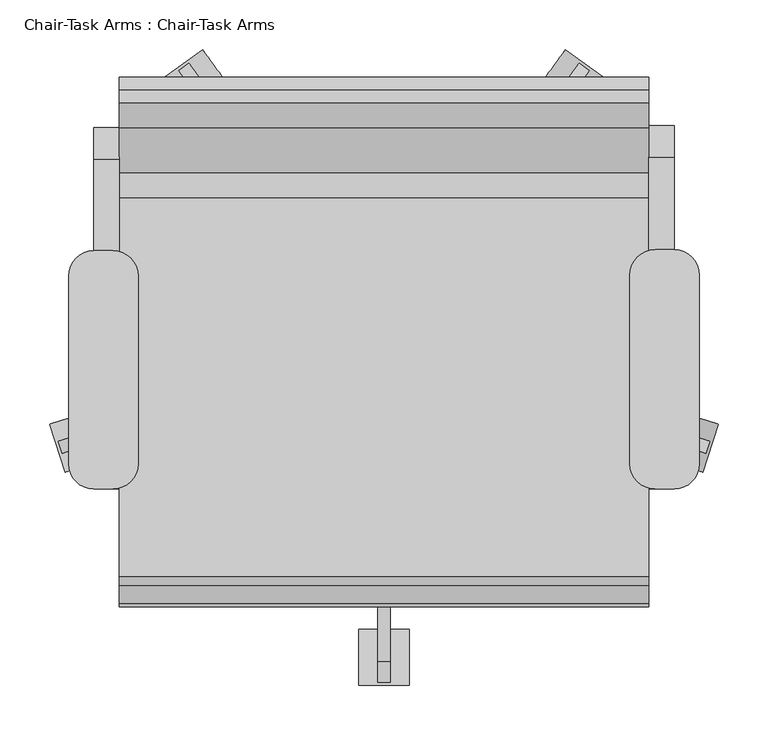
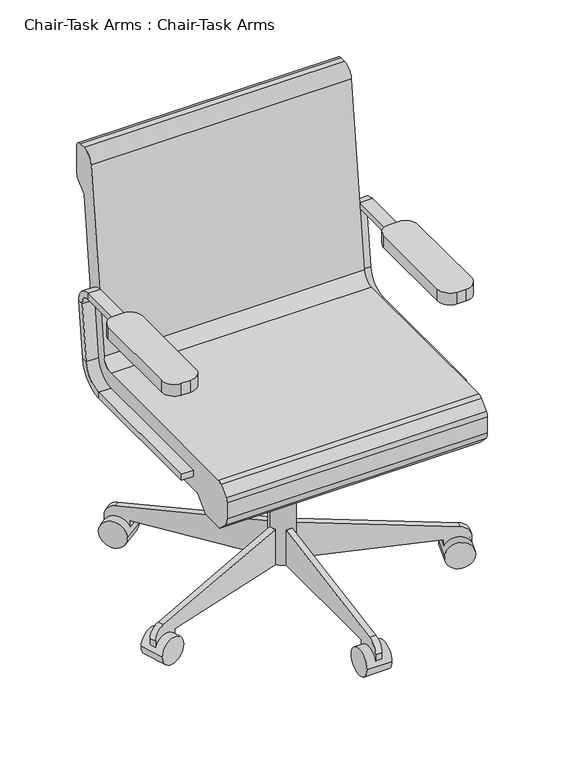
"""IFC4 building model written with IfcOpenShell, lengths in millimetres: furniture geometry, Chair-Task Arms : Chair-Task Arms."""

from ifc_helpers import new_model, si_unit, point, frame, frame_2d, origin, place, context, project, spatial, polyline, circle_curve, trimmed, segment, composite_curve, outline, extrude, source, transform, mapped, element, save
from ifc_brep_helpers import plane_surface, cylinder_surface, revolved_surface, advanced_brep


def chair_task_arms_chair_task_arms_83a3c27c(model_context):
    return source(origin(), model_context, "Body", "SolidModel", [
        extrude(outline(composite_curve([segment(trimmed(circle_curve(frame_2d((126.2050455, 482.6)), 25.4), [point((126.2050455, 457.2))], [point((151.4310708, 479.6322323))], True, "CARTESIAN"), True, "CONTINUOUS"), segment(polyline([(151.4310708, 479.6322323), (196.9528985, 866.5677677)]), True, "CONTINUOUS"), segment(trimmed(circle_curve(frame_2d((222.1789239, 863.6)), 25.4), [point((196.9528985, 866.5677677))], [point((222.1789239, 889.0))], False, "CARTESIAN"), True, "CONTINUOUS"), segment(polyline([(222.1789239, 889.0), (235.0540984, 889.0)]), True, "CONTINUOUS"), segment(trimmed(circle_curve(frame_2d((235.0540984, 876.3)), 12.7), [point((235.0540984, 889.0))], [point((247.7540984, 876.3))], False, "CARTESIAN"), True, "CONTINUOUS"), segment(polyline([(247.7540984, 876.3), (247.7540984, 818.0605122)]), True, "CONTINUOUS"), segment(trimmed(circle_curve(frame_2d((235.0540984, 818.0605122)), 12.7), [point((247.7540984, 818.0605122))], [point((244.0343545, 809.0802561))], False, "CARTESIAN"), True, "CONTINUOUS"), segment(polyline([(244.0343545, 809.0802561), (222.3540984, 787.4), (182.7870738, 451.0802913)]), True, "CONTINUOUS"), segment(trimmed(circle_curve(frame_2d((107.1089978, 459.9835944)), 76.2), [point((182.7870738, 451.0802913))], [point((107.1089978, 383.7835944))], False, "CARTESIAN"), True, "CONTINUOUS"), segment(polyline([(107.1089978, 383.7835944), (-181.0744602, 383.7835944), (-209.4470284, 355.6), (-260.2470284, 355.6), (-278.2663256, 373.7401184)]), True, "CONTINUOUS"), segment(trimmed(circle_curve(frame_2d((-260.2459016, 391.6405184)), 25.4), [point((-278.2663256, 373.7401184))], [point((-285.6459016, 391.6405184))], False, "CARTESIAN"), True, "CONTINUOUS"), segment(polyline([(-285.6459016, 391.6405184), (-285.6459016, 426.6837879)]), True, "CONTINUOUS"), segment(trimmed(circle_curve(frame_2d((-272.9459016, 426.6837879)), 12.7), [point((-285.6459016, 426.6837879))], [point((-281.8961016, 435.6939999))], False, "CARTESIAN"), True, "CONTINUOUS"), segment(polyline([(-281.8961016, 435.6939999), (-263.9604301, 453.510212)]), True, "CONTINUOUS"), segment(trimmed(circle_curve(frame_2d((-255.0102301, 444.5)), 12.7), [point((-263.9604301, 453.510212))], [point((-255.0102301, 457.2))], False, "CARTESIAN"), True, "CONTINUOUS"), segment(polyline([(-255.0102301, 457.2), (126.2050455, 457.2)]), True, "CONTINUOUS")], self_intersect=False)), frame((-125.7091803, 0.0, 0.0), z_axis=(1.0, 0.0, 0.0), x_axis=(0.0, 1.0, 0.0)), (0.0, 0.0, 1.0), 533.4),
        extrude(outline(polyline([(-69.7459016, 383.7835944), (19.1540984, 383.7835944), (19.1540984, 283.0954134), (-18.9459016, 283.0954134), (-69.7459016, 371.0835944), (-69.7459016, 383.7835944)])), frame((90.1908197, 0.0, 0.0), z_axis=(1.0, 0.0, 0.0), x_axis=(0.0, 1.0, 0.0)), (0.0, 0.0, 1.0), 101.6),
        extrude(outline(composite_curve([segment(polyline([(-311.0459016, 53.5835944), (-311.0459016, 28.1835944), (-361.8459016, 28.1835944), (-361.8459016, 52.4866474)]), True, "CONTINUOUS"), segment(trimmed(circle_curve(frame_2d((-336.4459016, 52.4866474)), 25.4), [point((-361.8459016, 52.4866474))], [point((-340.8565654, 77.5007643))], False, "CARTESIAN"), True, "CONTINUOUS"), segment(polyline([(-340.8565654, 77.5007643), (-44.3459016, 129.7835944), (-18.9459016, 129.7835944), (-18.9459016, 53.5835944), (-311.0459016, 53.5835944)]), True, "CONTINUOUS")], self_intersect=False)), frame((134.6408197, 0.0, 0.0), z_axis=(1.0, 0.0, 0.0), x_axis=(0.0, 1.0, 0.0)), (0.0, 0.0, 1.0), 12.7),
        extrude(outline(composite_curve([segment(trimmed(circle_curve(frame_2d((-336.4459016, 28.1835944)), 28.2002727), [point((-308.2456289, 28.1835944))], [point((-364.6461744, 28.1835944))], False, "CARTESIAN"), True, "CONTINUOUS"), segment(trimmed(circle_curve(frame_2d((-336.4459016, 28.1835944)), 28.2002727), [point((-364.6461744, 28.1835944))], [point((-308.2456289, 28.1835944))], False, "CARTESIAN"), True, "CONTINUOUS")], self_intersect=False)), frame((115.5908197, 0.0, 0.0), z_axis=(1.0, 0.0, 0.0), x_axis=(0.0, 1.0, 0.0)), (0.0, 0.0, 1.0), 50.8),
        extrude(outline(composite_curve([segment(polyline([(-25.4, 0.0), (-25.4, -292.1), (-101.6, -292.1), (-101.6, -266.7), (-49.3171699, 29.8106637)]), True, "CONTINUOUS"), segment(trimmed(circle_curve(frame_2d((-24.303053, 25.4)), 25.4), [point((-49.3171699, 29.8106637))], [point((-24.303053, 50.8000001))], False, "CARTESIAN"), True, "CONTINUOUS"), segment(polyline([(-24.303053, 50.8000001), (0.0, 50.8000001), (0.0, 0.0), (-25.4, 0.0)]), True, "CONTINUOUS")], self_intersect=False)), frame((-134.8505308, -115.2489746, 28.1835944), z_axis=(-0.3090169943749487, 0.9510565162951532, 0.0), x_axis=(0.0, 0.0, -1.0)), (0.0, 0.0, 1.0), 12.7),
        extrude(outline(composite_curve([segment(trimmed(circle_curve(frame_2d((0.0, 28.2002727)), 28.2002727), [point((0.0, 56.4005454))], [point((0.0, 0.0))], False, "CARTESIAN"), True, "CONTINUOUS"), segment(trimmed(circle_curve(frame_2d((0.0, 28.2002727)), 28.2002727), [point((0.0, 0.0))], [point((0.0, 56.4005454))], False, "CARTESIAN"), True, "CONTINUOUS")], self_intersect=False)), frame((-179.9406457, -149.9299964, 28.1835944), z_axis=(-0.3090169943749487, 0.9510565162951532, 0.0), x_axis=(0.0, 0.0, 1.0)), (0.0, 0.0, 1.0), 50.8),
        extrude(outline(composite_curve([segment(polyline([(-25.4, 0.0), (-25.4, -292.1), (-101.6, -292.1), (-101.6, -266.6999999), (-49.3171699, 29.8106637)]), True, "CONTINUOUS"), segment(trimmed(circle_curve(frame_2d((-24.303053, 25.3999999)), 25.4), [point((-49.3171699, 29.8106637))], [point((-24.303053, 50.8))], False, "CARTESIAN"), True, "CONTINUOUS"), segment(polyline([(-24.303053, 50.8), (0.0, 50.8), (0.0, 0.0), (-25.4, 0.0)]), True, "CONTINUOUS")], self_intersect=False)), frame((-35.8385104, 213.6355261, 28.1835944), z_axis=(0.8090169943749459, 0.5877852522924754, 0.0), x_axis=(0.0, 0.0, -1.0)), (0.0, 0.0, 1.0), 12.7),
        extrude(outline(composite_curve([segment(trimmed(circle_curve(frame_2d((0.0, 28.2002726)), 28.2002727), [point((0.0, 56.4005454))], [point((0.0, 0.0))], False, "CARTESIAN"), True, "CONTINUOUS"), segment(trimmed(circle_curve(frame_2d((0.0, 28.2002726)), 28.2002727), [point((0.0, 0.0))], [point((0.0, 56.4005454))], False, "CARTESIAN"), True, "CONTINUOUS")], self_intersect=False)), frame((-82.755734, 245.8017485, 28.1835944), z_axis=(0.8090169943749458, 0.5877852522924754, 0.0), x_axis=(0.0, 0.0, 1.0)), (0.0, 0.0, 1.0), 50.8),
        extrude(outline(composite_curve([segment(polyline([(25.4, 0.0), (0.0, 0.0), (0.0, 50.8), (24.303053, 50.8)]), True, "CONTINUOUS"), segment(trimmed(circle_curve(frame_2d((24.303053, 25.3999999)), 25.4), [point((24.303053, 50.8))], [point((49.3171699, 29.8106637))], False, "CARTESIAN"), True, "CONTINUOUS"), segment(polyline([(49.3171699, 29.8106637), (101.6, -266.7), (101.6, -292.1), (25.4, -292.1), (25.4, 0.0)]), True, "CONTINUOUS")], self_intersect=False)), frame((317.8201498, 213.6355261, 28.1835944), z_axis=(-0.8090169943749499, 0.5877852522924699, 0.0), x_axis=(0.0, 0.0, 1.0)), (0.0, 0.0, 1.0), 12.7),
        extrude(outline(composite_curve([segment(trimmed(circle_curve(frame_2d((0.0, 28.2002726)), 28.2002727), [point((0.0, 56.4005454))], [point((0.0, 0.0))], False, "CARTESIAN"), True, "CONTINUOUS"), segment(trimmed(circle_curve(frame_2d((0.0, 28.2002726)), 28.2002727), [point((0.0, 0.0))], [point((0.0, 56.4005454))], False, "CARTESIAN"), True, "CONTINUOUS")], self_intersect=False)), frame((364.7373733, 245.8017485, 28.1835944), z_axis=(-0.8090169943749499, 0.5877852522924699, 0.0), x_axis=(0.0, 0.0, -1.0)), (0.0, 0.0, 1.0), 50.8),
        extrude(outline(composite_curve([segment(polyline([(25.4, 0.0), (0.0, 0.0), (0.0, 50.8), (24.303053, 50.8)]), True, "CONTINUOUS"), segment(trimmed(circle_curve(frame_2d((24.303053, 25.4)), 25.4), [point((24.303053, 50.8))], [point((49.3171699, 29.8106636))], False, "CARTESIAN"), True, "CONTINUOUS"), segment(polyline([(49.3171699, 29.8106636), (101.6, -266.7), (101.6, -292.1), (25.4, -292.1), (25.4, 0.0)]), True, "CONTINUOUS")], self_intersect=False)), frame((416.8321702, -115.2489746, 28.1835944), z_axis=(0.3090169943749423, 0.9510565162951553, 0.0), x_axis=(0.0, 0.0, 1.0)), (0.0, 0.0, 1.0), 12.7),
        extrude(outline(composite_curve([segment(trimmed(circle_curve(frame_2d((0.0, 28.2002728)), 28.2002727), [point((0.0, 56.4005455))], [point((0.0, 0.0))], False, "CARTESIAN"), True, "CONTINUOUS"), segment(trimmed(circle_curve(frame_2d((0.0, 28.2002728)), 28.2002727), [point((0.0, 0.0))], [point((0.0, 56.4005455))], False, "CARTESIAN"), True, "CONTINUOUS")], self_intersect=False)), frame((461.9222851, -149.9299964, 28.1835944), z_axis=(0.3090169943749423, 0.9510565162951553, 0.0), x_axis=(0.0, 0.0, -1.0)), (0.0, 0.0, 1.0), 50.8),
        extrude(outline(composite_curve([segment(trimmed(circle_curve(frame_2d((140.9908197, -18.9459016)), 25.4), [point((115.5908197, -18.9459016))], [point((166.3908197, -18.9459016))], False, "CARTESIAN"), True, "CONTINUOUS"), segment(trimmed(circle_curve(frame_2d((140.9908197, -18.9459016)), 25.4), [point((166.3908197, -18.9459016))], [point((115.5908197, -18.9459016))], False, "CARTESIAN"), True, "CONTINUOUS")], self_intersect=False)), frame((0.0, 0.0, 53.5835944), z_axis=(0.0, 0.0, 1.0), x_axis=(1.0, 0.0, 0.0)), (0.0, 0.0, 1.0), 330.5914056),
        advanced_brep(
        [(433.0908197, -167.0319091, 425.45), (407.6908197, -167.0319091, 425.45), (407.6908197, -167.0319091, 412.75), (433.0908197, -167.0319091, 412.75), (433.0908197, 128.329278, 412.75), (433.0908197, 128.329278, 425.45), (407.6908197, 128.329278, 412.75), (407.6908197, 128.329278, 425.45), (433.0908197, 185.0878351, 463.2225227), (433.0908197, 172.4748224, 464.7064065), (407.6908197, 185.0878351, 463.2225227), (407.6908197, 172.4748224, 464.7064065), (433.0908197, 198.884043, 580.4902904), (433.0908197, 186.2710303, 581.9741742), (407.6908197, 198.884043, 580.4902904), (407.6908197, 186.2710303, 581.9741742), (433.0908197, 167.3515113, 615.95), (433.0908197, 167.3515113, 603.25), (407.6908197, 167.3515113, 615.95), (407.6908197, 167.3515113, 603.25), (433.0908197, -18.9459016, 603.25), (433.0908197, -18.9459016, 615.95), (407.6908197, -18.9459016, 615.95), (407.6908197, -18.9459016, 603.25)],
        [
            (0, 1),
            (1, 2),
            (2, 3),
            (3, 0),
            (3, 4),
            (4, 5),
            (5, 0),
            (2, 6),
            (6, 4),
            (1, 7),
            (7, 6),
            (5, 7),
            (8, 9),
            (9, 5, circle_curve(frame((433.0908197, 128.329278, 469.9), z_axis=(-1.0, 0.0, 0.0), x_axis=(0.0, 0.0, -1.0)), 44.45)),
            (4, 8, circle_curve(frame((433.0908197, 128.329278, 469.9), z_axis=(1.0, 0.0, 0.0), x_axis=(0.0, 0.0, -1.0)), 57.15)),
            (10, 8),
            (6, 10, circle_curve(frame((407.6908197, 128.329278, 469.9), z_axis=(1.0, 0.0, 0.0), x_axis=(0.0, 0.0, -1.0)), 57.15)),
            (11, 10),
            (7, 11, circle_curve(frame((407.6908197, 128.329278, 469.9), z_axis=(1.0, 0.0, 0.0), x_axis=(0.0, 0.0, -1.0)), 44.45)),
            (9, 11),
            (8, 12),
            (12, 13),
            (13, 9),
            (10, 14),
            (14, 12),
            (11, 15),
            (15, 14),
            (13, 15),
            (16, 17),
            (17, 13, circle_curve(frame((433.0908197, 167.3515113, 584.2), z_axis=(-1.0, 0.0, 0.0), x_axis=(0.0, 0.9931506043228767, -0.1168412475673929)), 19.05)),
            (12, 16, circle_curve(frame((433.0908197, 167.3515113, 584.2), z_axis=(1.0, 0.0, 0.0), x_axis=(0.0, 0.9931506043228767, -0.1168412475673929)), 31.75)),
            (18, 16),
            (14, 18, circle_curve(frame((407.6908197, 167.3515113, 584.2), z_axis=(1.0, 0.0, 0.0), x_axis=(0.0, 0.9931506043228767, -0.1168412475673929)), 31.75)),
            (19, 18),
            (15, 19, circle_curve(frame((407.6908197, 167.3515113, 584.2), z_axis=(1.0, 0.0, 0.0), x_axis=(0.0, 0.9931506043228767, -0.1168412475673929)), 19.05)),
            (17, 19),
            (20, 21),
            (21, 22),
            (22, 23),
            (23, 20),
            (16, 21),
            (20, 17),
            (18, 22),
            (19, 23),
        ],
        [
            plane_surface(frame((406.191788, -167.0319091, 419.1), z_axis=(0.0, -1.0, 0.0), x_axis=(0.0, 0.0, -1.0))),
            plane_surface(frame((433.0908197, -167.0319091, 425.45), z_axis=(1.0, 0.0, 0.0), x_axis=(0.0, 1.0, 0.0))),
            plane_surface(frame((433.0908197, -167.0319091, 412.75), z_axis=(0.0, 0.0, -1.0), x_axis=(0.0, 1.0, 0.0))),
            plane_surface(frame((407.6908197, -167.0319091, 412.75), z_axis=(-1.0, 0.0, 0.0), x_axis=(0.0, 1.0, 0.0))),
            plane_surface(frame((407.6908197, -167.0319091, 425.45), z_axis=(0.0, 0.0, 1.0), x_axis=(0.0, 1.0, 0.0))),
            plane_surface(frame((433.0908197, 128.329278, 469.9), z_axis=(1.0, 0.0, 0.0), x_axis=(0.0, 0.0, -1.0))),
            cylinder_surface(frame((420.3908197, 128.329278, 469.9), z_axis=(-1.0, 0.0, 0.0), x_axis=(0.0, 0.0, -1.0)), 57.15),
            plane_surface(frame((407.6908197, 128.329278, 469.9), z_axis=(-1.0, 0.0, 0.0), x_axis=(0.0, 0.0, -1.0))),
            revolved_surface(polyline([(407.6908197, 128.329278, 425.45), (433.0908197, 128.329278, 425.45)]), (420.3908197, 128.329278, 469.9), (-1.0, 0.0, 0.0)),
            plane_surface(frame((433.0908197, 172.4748224, 464.7064065), z_axis=(1.0, 0.0, 0.0), x_axis=(0.0, 0.11684124756738626, 0.9931506043228775))),
            plane_surface(frame((433.0908197, 185.0878351, 463.2225227), z_axis=(0.0, 0.9931506043228775, -0.11684124756738655), x_axis=(0.0, 0.11684124756738655, 0.9931506043228775))),
            plane_surface(frame((407.6908197, 185.0878351, 463.2225227), z_axis=(-1.0, 0.0, 0.0), x_axis=(0.0, 0.11684124756738626, 0.9931506043228775))),
            plane_surface(frame((407.6908197, 172.4748224, 464.7064065), z_axis=(0.0, -0.9931506043228775, 0.11684124756738626), x_axis=(0.0, 0.11684124756738626, 0.9931506043228775))),
            plane_surface(frame((433.0908197, 167.3515113, 584.2), z_axis=(1.0, 0.0, 0.0), x_axis=(0.0, 0.9931506043228767, -0.1168412475673929))),
            cylinder_surface(frame((420.3908197, 167.3515113, 584.2), z_axis=(-1.0, 0.0, 0.0), x_axis=(0.0, 0.9931506043228767, -0.1168412475673929)), 31.75),
            plane_surface(frame((407.6908197, 167.3515113, 584.2), z_axis=(-1.0, 0.0, 0.0), x_axis=(0.0, 0.9931506043228767, -0.1168412475673929))),
            revolved_surface(polyline([(407.6908197, 186.2710303123508, 581.9741742338412), (433.0908197, 186.2710303123508, 581.9741742338412)]), (420.3908197, 167.3515113, 584.2), (-1.0, 0.0, 0.0)),
            plane_surface(frame((406.191788, -18.9459016, 609.6), z_axis=(0.0, -1.0, 0.0), x_axis=(0.0, 0.0, 1.0))),
            plane_surface(frame((433.0908197, 167.3515113, 603.25), z_axis=(1.0, 0.0, 0.0), x_axis=(0.0, -1.0, 0.0))),
            plane_surface(frame((433.0908197, 167.3515113, 615.95), z_axis=(0.0, 0.0, 1.0), x_axis=(0.0, -1.0, 0.0))),
            plane_surface(frame((407.6908197, 167.3515113, 615.95), z_axis=(-1.0, 0.0, 0.0), x_axis=(0.0, -1.0, 0.0))),
            plane_surface(frame((407.6908197, 167.3515113, 603.25), z_axis=(0.0, 0.0, -1.0), x_axis=(0.0, -1.0, 0.0))),
        ],
        [
            (0, [[1, 2, 3, 4]]),
            (1, [[5, 6, 7, -4]]),
            (2, [[8, 9, -5, -3]]),
            (3, [[10, 11, -8, -2]]),
            (4, [[-7, 12, -10, -1]]),
            (5, [[13, 14, -6, 15]]),
            (6, [[16, -15, -9, 17]]),
            (7, [[18, -17, -11, 19]]),
            (8, [[20, -19, -12, -14]]),
            (9, [[21, 22, 23, -13]]),
            (10, [[24, 25, -21, -16]]),
            (11, [[26, 27, -24, -18]]),
            (12, [[-23, 28, -26, -20]]),
            (13, [[29, 30, -22, 31]]),
            (14, [[32, -31, -25, 33]]),
            (15, [[34, -33, -27, 35]]),
            (16, [[36, -35, -28, -30]]),
            (17, [[37, 38, 39, 40]]),
            (18, [[41, -37, 42, -29]]),
            (19, [[43, -38, -41, -32]]),
            (20, [[44, -39, -43, -34]]),
            (21, [[-42, -40, -44, -36]]),
        ],
    ),
        advanced_brep(
        [(-151.1091803, -167.0319091, 412.75), (-125.7091803, -167.0319091, 412.75), (-125.7091803, -167.0319091, 425.45), (-151.1091803, -167.0319091, 425.45), (-151.1091803, 126.2388651, 425.45), (-151.1091803, 126.2388651, 412.75), (-125.7091803, 126.2388651, 425.45), (-125.7091803, 126.2388651, 412.75), (-151.1091803, 170.3844094, 464.7064065), (-151.1091803, 182.9974221, 463.2225227), (-125.7091803, 170.3844094, 464.7064065), (-125.7091803, 182.9974221, 463.2225227), (-151.1091803, 184.1806174, 581.9741742), (-151.1091803, 196.7936301, 580.4902904), (-125.7091803, 184.1806174, 581.9741742), (-125.7091803, 196.7936301, 580.4902904), (-151.1091803, 165.2610984, 603.25), (-151.1091803, 165.2610984, 615.95), (-125.7091803, 165.2610984, 603.25), (-125.7091803, 165.2610984, 615.95), (-151.1091803, -18.9459016, 615.95), (-151.1091803, -18.9459016, 603.25), (-125.7091803, -18.9459016, 603.25), (-125.7091803, -18.9459016, 615.95)],
        [
            (0, 1),
            (1, 2),
            (2, 3),
            (3, 0),
            (3, 4),
            (4, 5),
            (5, 0),
            (2, 6),
            (6, 4),
            (1, 7),
            (7, 6),
            (5, 7),
            (8, 9),
            (9, 5, circle_curve(frame((-151.1091803, 126.2388651, 469.9), z_axis=(-1.0, 0.0, 0.0), x_axis=(0.0, 0.0, -1.0)), 57.15)),
            (4, 8, circle_curve(frame((-151.1091803, 126.2388651, 469.9), z_axis=(1.0, 0.0, 0.0), x_axis=(0.0, 0.0, -1.0)), 44.45)),
            (10, 8),
            (6, 10, circle_curve(frame((-125.7091803, 126.2388651, 469.9), z_axis=(1.0, 0.0, 0.0), x_axis=(0.0, 0.0, -1.0)), 44.45)),
            (11, 10),
            (7, 11, circle_curve(frame((-125.7091803, 126.2388651, 469.9), z_axis=(1.0, 0.0, 0.0), x_axis=(0.0, 0.0, -1.0)), 57.15)),
            (9, 11),
            (8, 12),
            (12, 13),
            (13, 9),
            (10, 14),
            (14, 12),
            (11, 15),
            (15, 14),
            (13, 15),
            (16, 17),
            (17, 13, circle_curve(frame((-151.1091803, 165.2610984, 584.2), z_axis=(-1.0, 0.0, 0.0), x_axis=(0.0, 0.9931506043228768, -0.11684124756739202)), 31.75)),
            (12, 16, circle_curve(frame((-151.1091803, 165.2610984, 584.2), z_axis=(1.0, 0.0, 0.0), x_axis=(0.0, 0.9931506043228768, -0.11684124756739202)), 19.05)),
            (18, 16),
            (14, 18, circle_curve(frame((-125.7091803, 165.2610984, 584.2), z_axis=(1.0, 0.0, 0.0), x_axis=(0.0, 0.9931506043228768, -0.11684124756739202)), 19.05)),
            (19, 18),
            (15, 19, circle_curve(frame((-125.7091803, 165.2610984, 584.2), z_axis=(1.0, 0.0, 0.0), x_axis=(0.0, 0.9931506043228768, -0.11684124756739202)), 31.75)),
            (17, 19),
            (20, 21),
            (21, 22),
            (22, 23),
            (23, 20),
            (16, 21),
            (20, 17),
            (18, 22),
            (19, 23),
        ],
        [
            plane_surface(frame((-152.608212, -167.0319091, 419.1), z_axis=(0.0, -1.0, 0.0), x_axis=(0.0, 0.0, -1.0))),
            plane_surface(frame((-151.1091803, -167.0319091, 412.75), z_axis=(-1.0, 0.0, 0.0), x_axis=(0.0, 1.0, 0.0))),
            plane_surface(frame((-151.1091803, -167.0319091, 425.45), z_axis=(0.0, 0.0, 1.0), x_axis=(0.0, 1.0, 0.0))),
            plane_surface(frame((-125.7091803, -167.0319091, 425.45), z_axis=(1.0, 0.0, 0.0), x_axis=(0.0, 1.0, 0.0))),
            plane_surface(frame((-125.7091803, -167.0319091, 412.75), z_axis=(0.0, 0.0, -1.0), x_axis=(0.0, 1.0, 0.0))),
            plane_surface(frame((-151.1091803, 126.2388651, 469.9), z_axis=(-1.0, 0.0, 0.0), x_axis=(0.0, 0.0, -1.0))),
            revolved_surface(polyline([(-151.1091803, 126.2388651, 425.45), (-125.7091803, 126.2388651, 425.45)]), (-138.4091803, 126.2388651, 469.9), (-1.0, 0.0, 0.0)),
            plane_surface(frame((-125.7091803, 126.2388651, 469.9), z_axis=(1.0, 0.0, 0.0), x_axis=(0.0, 0.0, -1.0))),
            cylinder_surface(frame((-138.4091803, 126.2388651, 469.9), z_axis=(-1.0, 0.0, 0.0), x_axis=(0.0, 0.0, -1.0)), 57.15),
            plane_surface(frame((-151.1091803, 182.9974221, 463.2225227), z_axis=(-1.0, 0.0, 0.0), x_axis=(0.0, 0.1168412475673856, 0.9931506043228776))),
            plane_surface(frame((-151.1091803, 170.3844094, 464.7064065), z_axis=(0.0, -0.9931506043228776, 0.1168412475673856), x_axis=(0.0, 0.1168412475673856, 0.9931506043228776))),
            plane_surface(frame((-125.7091803, 170.3844094, 464.7064065), z_axis=(1.0, 0.0, 0.0), x_axis=(0.0, 0.1168412475673856, 0.9931506043228776))),
            plane_surface(frame((-125.7091803, 182.9974221, 463.2225227), z_axis=(0.0, 0.9931506043228776, -0.1168412475673856), x_axis=(0.0, 0.1168412475673856, 0.9931506043228776))),
            plane_surface(frame((-151.1091803, 165.2610984, 584.2), z_axis=(-1.0, 0.0, 0.0), x_axis=(0.0, 0.9931506043228768, -0.11684124756739202))),
            revolved_surface(polyline([(-151.1091803, 184.1806174123508, 581.9741742338413), (-125.7091803, 184.1806174123508, 581.9741742338413)]), (-138.4091803, 165.2610984, 584.2), (-1.0, 0.0, 0.0)),
            plane_surface(frame((-125.7091803, 165.2610984, 584.2), z_axis=(1.0, 0.0, 0.0), x_axis=(0.0, 0.9931506043228768, -0.11684124756739202))),
            cylinder_surface(frame((-138.4091803, 165.2610984, 584.2), z_axis=(-1.0, 0.0, 0.0), x_axis=(0.0, 0.9931506043228768, -0.11684124756739202)), 31.75),
            plane_surface(frame((-152.608212, -18.9459016, 609.6), z_axis=(0.0, -1.0, 0.0), x_axis=(0.0, 0.0, 1.0))),
            plane_surface(frame((-151.1091803, 165.2610984, 615.95), z_axis=(-1.0, 0.0, 0.0), x_axis=(0.0, -1.0, 0.0))),
            plane_surface(frame((-151.1091803, 165.2610984, 603.25), z_axis=(0.0, 0.0, -1.0), x_axis=(0.0, -1.0, 0.0))),
            plane_surface(frame((-125.7091803, 165.2610984, 603.25), z_axis=(1.0, 0.0, 0.0), x_axis=(0.0, -1.0, 0.0))),
            plane_surface(frame((-125.7091803, 165.2610984, 615.95), z_axis=(0.0, 0.0, 1.0), x_axis=(0.0, -1.0, 0.0))),
        ],
        [
            (0, [[1, 2, 3, 4]]),
            (1, [[5, 6, 7, -4]]),
            (2, [[8, 9, -5, -3]]),
            (3, [[10, 11, -8, -2]]),
            (4, [[-7, 12, -10, -1]]),
            (5, [[13, 14, -6, 15]]),
            (6, [[16, -15, -9, 17]]),
            (7, [[18, -17, -11, 19]]),
            (8, [[20, -19, -12, -14]]),
            (9, [[21, 22, 23, -13]]),
            (10, [[24, 25, -21, -16]]),
            (11, [[26, 27, -24, -18]]),
            (12, [[-23, 28, -26, -20]]),
            (13, [[29, 30, -22, 31]]),
            (14, [[32, -31, -25, 33]]),
            (15, [[34, -33, -27, 35]]),
            (16, [[36, -35, -28, -30]]),
            (17, [[37, 38, 39, 40]]),
            (18, [[41, -37, 42, -29]]),
            (19, [[43, -38, -41, -32]]),
            (20, [[44, -39, -43, -34]]),
            (21, [[-42, -40, -44, -36]]),
        ],
    ),
        extrude(outline(composite_curve([segment(trimmed(circle_curve(frame_2d((433.0908197, 48.8028048)), 25.4), [point((433.0908197, 74.2028048))], [point((458.4908197, 48.8028048))], False, "CARTESIAN"), True, "CONTINUOUS"), segment(polyline([(458.4908197, 48.8028048), (458.4908197, -141.6319091)]), True, "CONTINUOUS"), segment(trimmed(circle_curve(frame_2d((433.0908197, -141.6319091)), 25.4), [point((458.4908197, -141.6319091))], [point((433.0908197, -167.0319091))], False, "CARTESIAN"), True, "CONTINUOUS"), segment(polyline([(433.0908197, -167.0319091), (414.0408197, -167.0319091)]), True, "CONTINUOUS"), segment(trimmed(circle_curve(frame_2d((414.0408197, -141.6319091)), 25.4), [point((414.0408197, -167.0319091))], [point((388.6408197, -141.6319091))], False, "CARTESIAN"), True, "CONTINUOUS"), segment(polyline([(388.6408197, -141.6319091), (388.6408197, 48.8028048)]), True, "CONTINUOUS"), segment(trimmed(circle_curve(frame_2d((414.0408197, 48.8028048)), 25.4), [point((388.6408197, 48.8028048))], [point((414.0408197, 74.2028048))], False, "CARTESIAN"), True, "CONTINUOUS"), segment(polyline([(414.0408197, 74.2028048), (433.0908197, 74.2028048)]), True, "CONTINUOUS")], self_intersect=False)), frame((0.0, 0.0, 596.9), z_axis=(0.0, 0.0, 1.0), x_axis=(1.0, 0.0, 0.0)), (0.0, 0.0, 1.0), 25.4),
        extrude(outline(composite_curve([segment(trimmed(circle_curve(frame_2d((-132.0591803, 47.7575984)), 25.4), [point((-132.0591803, 73.1575984))], [point((-106.6591803, 47.7575984))], False, "CARTESIAN"), True, "CONTINUOUS"), segment(polyline([(-106.6591803, 47.7575984), (-106.6591803, -141.6319091)]), True, "CONTINUOUS"), segment(trimmed(circle_curve(frame_2d((-132.0591803, -141.6319091)), 25.4), [point((-106.6591803, -141.6319091))], [point((-132.0591803, -167.0319091))], False, "CARTESIAN"), True, "CONTINUOUS"), segment(polyline([(-132.0591803, -167.0319091), (-151.1091803, -167.0319091)]), True, "CONTINUOUS"), segment(trimmed(circle_curve(frame_2d((-151.1091803, -141.6319091)), 25.4), [point((-151.1091803, -167.0319091))], [point((-176.5091803, -141.6319091))], False, "CARTESIAN"), True, "CONTINUOUS"), segment(polyline([(-176.5091803, -141.6319091), (-176.5091803, 47.7575984)]), True, "CONTINUOUS"), segment(trimmed(circle_curve(frame_2d((-151.1091803, 47.7575984)), 25.4), [point((-176.5091803, 47.7575984))], [point((-151.1091803, 73.1575984))], False, "CARTESIAN"), True, "CONTINUOUS"), segment(polyline([(-151.1091803, 73.1575984), (-132.0591803, 73.1575984)]), True, "CONTINUOUS")], self_intersect=False)), frame((0.0, 0.0, 596.9), z_axis=(0.0, 0.0, 1.0), x_axis=(1.0, 0.0, 0.0)), (0.0, 0.0, 1.0), 25.4),
    ])


if __name__ == "__main__":
    model = new_model("IFC4")
    model_context = context("Model", 3, world=origin())
    ifc_project = project(units=[si_unit("LENGTHUNIT", "METRE", prefix="MILLI")], contexts=[model_context])
    site = spatial("IfcSite", under=ifc_project)
    building = spatial("IfcBuilding", under=site)
    placement = place(None, origin())
    chair_task_arms_chair_task_arms_shape = chair_task_arms_chair_task_arms_83a3c27c(model_context)
    element("IfcFurniture", 1, ObjectType="Chair-Task Arms : Chair-Task Arms", at=placement, inside=building, context=model_context, shape_type="MappedRepresentation", body=[
        mapped(chair_task_arms_chair_task_arms_shape, transform((0.0, 0.0, 0.0), x_axis=(1.0, 0.0, 0.0), y_axis=(0.0, 1.0, 0.0), z_axis=(0.0, 0.0, 1.0))),
    ])
    save(model, "model.ifc")

# Revit data of these elements
# Type "Chair-Task Arms : Chair-Task Arms"
#   Assembly Code = "E2020200"
#   Base Material = Plastic, Opaque Black
#   Caster Material = Plastic, Opaque Black
#   Seat/Back Material = Textile - Slate Blue
#   Default Elevation = 0
# Element 1 (IfcFurniture, "Chair-Task Arms : Chair-Task Arms")
#   Materials on its faces: "Plastic, Opaque Black", "Textile - Slate Blue"
# Materials
#   "Plastic, Opaque Black": class "Plastic", colour RGB 0 0 0, transparency 0, Description = "Plastic, generic, opaque black", Cost = 0
#   "Textile - Slate Blue": class "Fabric", colour RGB 98 102 118, transparency 0
